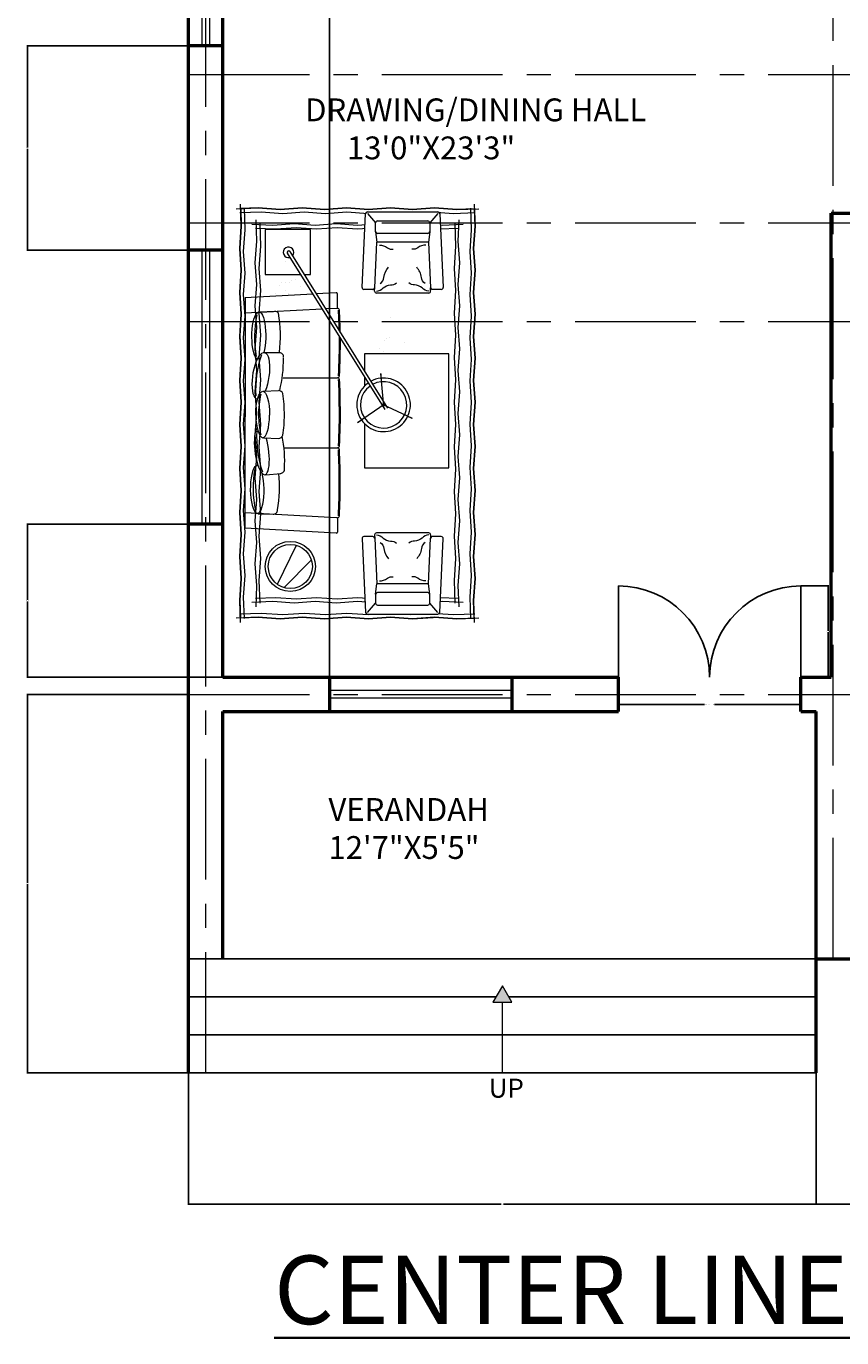
# Model space of a CAD drawing. Units: inches. Extents: x 10696 to 11614, y 5787 to 6498.
# Tile 6 of 9: x 11123 to 11338, y 5787 to 6132. Entities that reach past the tile are written whole.
import ezdxf

# ---------------------------------------------------------------- set-up
doc = ezdxf.new("R2010")
doc.units = ezdxf.units.IN
doc.set_wipeout_variables(frame=1)
doc.linetypes.add('CENTER', pattern=[50.8, 31.75, -6.35, 6.35, -6.35])
for name, color, linetype, lineweight in [('A-ANNO-DIMS', 2, 'Continuous', 18), ('A-ANNO-SYMB', 2, 'Continuous', 18), ('A-ANNO-TITL', 7, 'Continuous', 35), ('A-AREA-IDEN', 7, 'Continuous', 25), ('A-DOOR', 3, 'Continuous', 25), ('A-FLOR', 7, 'Continuous', 25), ('A-FLOR-STRS', 7, 'Continuous', 25), ('A-FURN', 8, 'Continuous', 18), ('A-GLAZ', 4, 'Continuous', 20), ('A-GRID', 1, 'CENTER', 18), ('A-WALL', 7, 'Continuous', 50)]:
    doc.layers.add(name, color=color, linetype=linetype, lineweight=lineweight)
doc.styles.get("Standard").update_dxf_attribs({"font": 'arial.ttf'})
doc.dimstyles.get("Standard").update_dxf_attribs({"dimtxt": 0.18, "dimasz": 0.18, "dimexe": 0.18, "dimexo": 0.0625, "dimgap": 0.09, "dimtad": 0, "dimtih": 1, "dimtoh": 1, "dimdec": 4, "dimzin": 0, "dimdsep": 46, "dimtxsty": 'Standard', "dimcen": 0.09, "dimadec": 0, "dimazin": 0, "dimtfac": 1, "dimtdec": 4, "dimtofl": 0, "dimtmove": 0, "dimatfit": 3, "dimfxl": 1, "dimtolj": 1, "dimtzin": 0, "dimarcsym": 0})

# ---------------------------------------------------------------- blocks, each defined once
blk = doc.blocks.new('A$C7590614E')
for p, q in [((220, 4135), (46, 4129)), ((46, 4129), (52, 3952)), ((46, 4129), (46, 4129)), ((440, 4119), (220, 4135)), ((660, 4135), (440, 4119)), ((881, 4119), (660, 4135)), ((1101, 4135), (881, 4119)), ((1321, 4119), (1101, 4135)), ((1541, 4135), (1321, 4119)), ((1761, 4119), (1541, 4135)), ((1981, 4135), (1761, 4119)), ((2202, 4119), (1981, 4135)), ((2379, 4126), (2202, 4119)), ((2385, 3952), (2379, 4126)), ((52, 3952), (36, 3732)), ((2369, 3732), (2385, 3952)), ((36, 3732), (52, 3513)), ((2385, 3513), (2369, 3732)), ((496, 3597), (496, 3597)), ((596, 3620), (596, 3620)), ((52, 3513), (36, 3293)), ((553, 3416), (553, 3416)), ((592, 3420), (592, 3420)), ((2369, 3293), (2385, 3513)), ((36, 3293), (52, 3074)), ((765, 3275), (91, 3238)), ((392, 3284), (392, 3284)), ((436, 3366), (436, 3366)), ((454, 3393), (454, 3393)), ((492, 3396), (492, 3396)), ((492, 3308), (492, 3308)), ((526, 3286), (526, 3286)), ((536, 3390), (536, 3390)), ((641, 3347), (641, 3347)), ((741, 3371), (741, 3371)), ((1000, 3288), (799, 3277)), ((1011, 3134), (1011, 3278)), ((2385, 3074), (2369, 3293)), ((91, 3238), (91, 2051)), ((91, 3161), (91, 2051)), ((426, 3262), (426, 3262)), ((52, 3074), (37, 2858)), ((859, 3125), (91, 3084)), ((236, 3098), (385, 3104)), ((374, 3100), (240, 3093)), ((332, 3098), (253, 3094)), ((1010, 3133), (893, 3127)), ((1538, 3041), (1538, 3041)), ((2369, 2854), (2385, 3074)), ((37, 2858), (52, 2635)), ((1479, 2810), (1479, 2810)), ((1496, 2837), (1496, 2837)), ((1535, 2840), (1535, 2840)), ((1683, 2791), (1683, 2791)), ((2385, 2635), (2369, 2854)), ((52, 2635), (36, 2415)), ((276, 2693), (435, 2692)), ((1434, 2729), (1434, 2729)), ((1469, 2706), (1469, 2706)), ((2369, 2415), (2385, 2635)), ((36, 2415), (52, 2196)), ((469, 2441), (1012, 2441)), ((2385, 2196), (2369, 2415)), ((275, 2308), (424, 2314)), ((52, 2196), (36, 1976)), ((2369, 1976), (2385, 2196)), ((36, 1976), (52, 1756)), ((91, 941), (91, 2051)), ((91, 941), (91, 2051)), ((2385, 1756), (2369, 1976)), ((275, 1842), (424, 1836)), ((52, 1756), (36, 1537)), ((478, 1742), (1012, 1742)), ((2369, 1537), (2385, 1756)), ((36, 1537), (52, 1317)), ((296, 1474), (445, 1487)), ((2385, 1317), (2369, 1537)), ((52, 1317), (36, 1098)), ((2369, 1098), (2385, 1317)), ((36, 1098), (52, 878)), ((1001, 1045), (91, 1095)), ((221, 1085), (370, 1080)), ((2385, 878), (2369, 1098)), ((1001, 891), (91, 941)), ((1010, 1045), (1001, 1045)), ((1011, 1045), (1011, 901)), ((52, 878), (36, 659)), ((2369, 659), (2385, 878)), ((36, 659), (52, 439)), ((2385, 439), (2369, 659)), ((52, 439), (36, 220)), ((2369, 220), (2385, 439)), ((36, 220), (43, 46)), ((2376, 43), (2369, 220)), ((43, 46), (220, 52)), ((220, 52), (440, 36)), ((440, 36), (660, 52)), ((660, 52), (881, 36)), ((881, 36), (1101, 52)), ((1101, 52), (1321, 36)), ((1321, 36), (1541, 52)), ((1541, 52), (1761, 36)), ((1761, 36), (1966, 51)), ((1966, 51), (1981, 52)), ((1981, 52), (2202, 36)), ((2202, 36), (2376, 43))]:
    blk.add_line(p, q)
at = {"linetype": 'ByBlock'}
for p, q in [((1474, 2154, 0), (1445, 2485, 0)), ((1474, 2154, 0), (1445, 2485, 0)), ((1450, 2427, 0), (1446, 2481, 0)), ((1487, 2182, 0), (1213, 1991, 0)), ((1487, 2182, 0), (1213, 1991, 0)), ((1456, 2179, 0), (1757, 2037, 0)), ((1456, 2179, 0), (1757, 2037, 0)), ((1261, 2025, 0), (1217, 1994, 0)), ((1705, 2062, 0), (1754, 2039, 0)), ((412, 381), (604, 770)), ((751, 626), (481, 348))]:
    blk.add_line(p, q, dxfattribs=at)
at = {"linetype": 'ByBlock', "flags": 128}
for points in [[(0, 4127), (220, 4135), (440, 4119), (660, 4135), (881, 4119), (1101, 4135), (1321, 4119), (1541, 4135), (1761, 4119), (1981, 4135), (2202, 4119), (2422, 4127)], [(44, 0), (36, 220), (52, 439), (36, 659), (52, 878), (36, 1098), (52, 1317), (36, 1537), (52, 1756), (36, 1976), (52, 2196), (36, 2415), (52, 2635), (36, 2854), (52, 3074), (36, 3293), (52, 3513), (36, 3732), (52, 3952), (44, 4172)], [(39, 4088), (252, 4096), (465, 4080), (678, 4096), (891, 4080), (1104, 4096), (1317, 4080), (1531, 4096), (1744, 4080), (1957, 4096), (2170, 4080), (2383, 4088)], [(83, 39), (75, 254), (91, 470), (75, 685), (91, 901), (75, 1116), (91, 1332), (75, 1547), (91, 1763), (75, 1978), (91, 2194), (75, 2409), (91, 2624), (75, 2840), (91, 3055), (75, 3271), (91, 3486), (75, 3702), (91, 3917), (83, 4133)], [(2339, 4133), (2347, 3917), (2331, 3702), (2347, 3486), (2331, 3271), (2347, 3055), (2331, 2840), (2347, 2624), (2331, 2409), (2347, 2194), (2331, 1978), (2347, 1763), (2331, 1547), (2347, 1332), (2331, 1116), (2347, 901), (2331, 685), (2347, 470), (2331, 254), (2339, 39)], [(2377, 4172), (2385, 3952), (2369, 3732), (2385, 3513), (2369, 3293), (2385, 3074), (2369, 2854), (2385, 2635), (2369, 2415), (2385, 2196), (2369, 1976), (2385, 1756), (2369, 1537), (2385, 1317), (2369, 1098), (2385, 878), (2369, 659), (2385, 439), (2369, 220), (2377, 0)], [(156, 3972), (367, 3964), (578, 3980), (789, 3964), (1000, 3980), (1211, 3964), (1422, 3980), (1633, 3964), (1844, 3980), (2055, 3964), (2266, 3972)], [(200, 156), (208, 370), (192, 584), (208, 799), (192, 1013), (208, 1228), (192, 1442), (208, 1657), (192, 1871), (208, 2086), (192, 2300), (208, 2515), (192, 2729), (208, 2944), (192, 3158), (208, 3373), (192, 3587), (208, 3802), (200, 4016)], [(194, 3933), (398, 3925), (601, 3941), (804, 3925), (1008, 3941), (1211, 3925), (1414, 3941), (1617, 3925), (1821, 3941), (2024, 3925), (2227, 3933)], [(239, 194), (231, 417), (247, 639), (231, 862), (247, 1084), (231, 1307), (247, 1529), (231, 1752), (247, 1975), (231, 2197), (247, 2420), (231, 2642), (247, 2865), (231, 3087), (247, 3310), (231, 3532), (247, 3755), (239, 3977)], [(2183, 3977), (2191, 3755), (2175, 3532), (2191, 3310), (2175, 3087), (2191, 2865), (2175, 2642), (2191, 2420), (2175, 2197), (2191, 1975), (2175, 1752), (2191, 1529), (2175, 1307), (2191, 1084), (2175, 862), (2191, 639), (2175, 417), (2183, 194)], [(2222, 4016), (2214, 3802), (2230, 3587), (2214, 3373), (2230, 3158), (2214, 2944), (2230, 2729), (2214, 2515), (2230, 2300), (2214, 2086), (2230, 1871), (2214, 1657), (2230, 1442), (2214, 1228), (2230, 1013), (2214, 799), (2230, 584), (2214, 370), (2222, 156)], [(2266, 200), (2055, 208), (1844, 192), (1633, 208), (1422, 192), (1211, 208), (1000, 192), (789, 208), (578, 192), (367, 208), (156, 200)], [(2227, 239), (2024, 247), (1821, 231), (1617, 247), (1414, 231), (1211, 247), (1008, 231), (804, 247), (601, 231), (398, 247), (194, 239)], [(2422, 44), (2202, 36), (1981, 52), (1761, 36), (1541, 52), (1321, 36), (1101, 52), (881, 36), (660, 52), (440, 36), (220, 52), (0, 44)], [(2383, 83), (2170, 75), (1957, 91), (1744, 75), (1531, 91), (1317, 75), (1104, 91), (891, 75), (678, 91), (465, 75), (252, 91), (39, 83)]]:
    blk.add_lwpolyline(points, dxfattribs=at)
at = {"linetype": 'ByBlock'}
blk.add_lwpolyline([(678, 3471), (741, 3471), (741, 3921), (291, 3921), (291, 3471), (643, 3471)], dxfattribs=at)
for points in [[(1282, 1984), (1282, 1541), (2122, 1541), (2122, 2681), (1282, 2681), (1282, 2504)], [(1282, 2447), (1282, 2359)]]:
    blk.add_lwpolyline(points)
at = {"linetype": 'ByBlock', "const_width": 10, "elevation": 0}
for points in [[(1450, 2427), (1446, 2481)], [(1261, 2025), (1217, 1994)], [(1705, 2062), (1754, 2039)]]:
    blk.add_lwpolyline(points, dxfattribs=at)
at = {"linetype": 'ByBlock'}
for radius in [250, 220]:
    blk.add_circle((541, 559), radius, dxfattribs=at)
for radius, start, end in [(52.4, 318.5939, 285.3184), (15, 31.9562, 211.9562)]:
    blk.add_arc((523, 3692), radius, start, end, dxfattribs=at)
for centre, radius, start, end in [((1001, 3278), 10, 0, 93.0128), ((1254, 2846), 1070, 168.034, 190.3551), ((-385, 2845), 798, 18.6145, 18.6419), ((387, 3061), 42.5, 33.8407, 92.0223), ((-822, 2855), 1265, 352.6106, 10.4711), ((1011, 3113), 20, 3.7459, 93.0128), ((-4595, 2788), 5626, 1.223, 3.3226), ((-4595, 2788), 5636, 1.0525, 3.3226), ((-4595, 2788), 5626, 356.669, 0.6303), ((-4595, 2788), 5636, 356.669, 0.4637), ((1265, 2321), 1070, 160.9121, 183.2331), ((431, 2650), 42.5, 352.6116, 84.9003), ((-796, 2619), 1269, 346.0345, 0.8134), ((1011, 2421), 20, 3.742, 91.3972), ((1011, 2461), 20, 271.3972, 356.2445), ((-2252, 2185), 3282, 359.485, 4.1508), ((-2252, 2185), 3292, 359.485, 4.1508), ((1293, 2055), 1070, 168.034, 179.2769), ((425, 2271), 42.5, 16.3929, 92.0223), ((-783, 2085), 1265, 359.2714, 9.0059), ((425, 2271), 42.5, 359.7336, 1.1068), ((-4089, 2069), 5120, 356.563, 0.9635), ((-4089, 2069), 5130, 356.563, 0.9635), ((1293, 2094), 1070, 181.3636, 191.966), ((-783, 2065), 1265, 350.9941, 0.1868), ((1275, 1851), 1070, 176.7669, 199.0879), ((425, 1879), 42.5, 267.9777, 343.6071), ((-780, 1606), 1265, 356.7804, 11.4363), ((425, 1879), 42.5, 358.8932, 0.2664), ((1011, 1762), 20, 268.6028, 356.258), ((1011, 1722), 20, 3.7555, 88.6028), ((-4697, 1393), 5727, 356.706, 3.3024), ((-4697, 1393), 5737, 356.706, 3.3024), ((1239, 1338), 1070, 169.6449, 191.966), ((-831, 1350), 1265, 349.6584, 6.1656), ((441, 1530), 42.5, 275.0997, 7.3884), ((-400, 1339), 798, 341.3581, 341.3855), ((371, 1122), 42.5, 267.9777, 0.2664), ((1011, 1065), 20, 266.9872, 356.2541), ((1001, 901), 10, 266.9872, 0)]:
    blk.add_arc(centre, radius, start, end)
at = {"extrusion": (0, 0, -1)}
for centre, major_axis, ratio, start_param, end_param in [((227, 2858), (2, 239), 0.289653, 3.343252, 8.61472), ((248, 2460), (35, 232), 0.342983, 3.115548, 8.511087), ((265, 2068), (2, 239), 0.289653, -1.56819, 1.564113)]:
    blk.add_ellipse(centre, major_axis=major_axis, ratio=ratio, start_param=start_param, end_param=end_param, dxfattribs=at)
at = {"linetype": 'ByBlock', "extrusion": (3.38184e-09, 2.26187e-09, 1)}
for major_axis, start_param, end_param in [((-219, -153, 0), 4.720612, 10.891434), ((-190, -132, 0), 4.729628, 10.883141)]:
    blk.add_ellipse((1472, 2171), major_axis=major_axis, ratio=1, start_param=start_param, end_param=end_param, dxfattribs=at)
for centre, major_axis, start_param, end_param in [((265, 2082), (-2, 239), 1.623473, 4.655635), ((257, 1711), (-31, 237), 0.253375, 5.250818), ((211, 1326), (-2, 239), -0.16583, 5.452765)]:
    blk.add_ellipse(centre, major_axis=major_axis, ratio=0.289653, start_param=start_param, end_param=end_param)
for points in [[(1941, 3334), (1941, 3305), (1940, 3297), (1936, 3292), (1929, 3287), (1929, 3287), (1919, 3286), (1838, 3286), (1732, 3286), (1653, 3286), (1475, 3286), (1400, 3286), (1392, 3288), (1387, 3292), (1383, 3298), (1382, 3305), (1382, 3311), (1383, 3317), (1383, 3329), (1383, 3336), (1378, 3327), (1372, 3323), (1366, 3322), (1359, 3322), (1271, 3323), (1263, 3328), (1263, 3328), (1259, 3334), (1258, 3341), (1258, 3341), (1292, 4079), (1294, 4086), (1297, 4091), (1297, 4091), (1310, 4096), (1316, 4096), (1326, 4096), (1336, 4096), (2002, 4096), (2014, 4096), (2026, 4091), (2032, 4079), (2032, 4070), (2066, 3341), (2061, 3328), (2061, 3328), (2048, 3322), (2028, 3322), (1992, 3322), (1958, 3322), (1951, 3324), (1945, 3327), (1944, 3329)], [(1941, 845), (1941, 874), (1940, 882), (1936, 887), (1929, 892), (1929, 892), (1919, 893), (1838, 893), (1732, 893), (1653, 893), (1475, 893), (1400, 893), (1392, 891), (1387, 887), (1383, 881), (1382, 874), (1382, 868), (1383, 862), (1383, 850), (1383, 843), (1378, 852), (1372, 856), (1366, 857), (1359, 857), (1271, 856), (1263, 851), (1263, 851), (1259, 845), (1258, 838), (1258, 838), (1292, 100), (1294, 93), (1297, 88), (1297, 88), (1310, 83), (1316, 83), (1326, 83), (1336, 83), (2002, 83), (2014, 83), (2026, 88), (2032, 100), (2032, 109), (2066, 838), (2061, 851), (2061, 851), (2048, 857), (2028, 857), (1992, 857), (1958, 857), (1951, 855), (1945, 852), (1944, 850)]]:
    blk.add_wipeout(points).translate(0, 0, 0)
at = {"linetype": 'ByBlock'}
for p, q in [((1258, 3341, 0), (1292, 4079, 0)), ((1310, 4096, 0), (2014, 4096, 0)), ((1310, 4078, 0), (1392, 3988, 0)), ((1310, 4078, 0), (1392, 3988, 0)), ((2014, 4078, 0), (1932, 3988, 0)), ((2014, 4078, 0), (1932, 3988, 0)), ((2032, 4079, 0), (2066, 3341, 0)), ((1392, 3898, 0), (1392, 3988, 0)), ((1392, 3898, 0), (1392, 3988, 0)), ((1410, 4006, 0), (1914, 4006, 0)), ((1410, 4006, 0), (1914, 4006, 0)), ((1932, 3988, 0), (1932, 3898, 0)), ((1932, 3988, 0), (1932, 3898, 0)), ((1392, 3898, 0), (1405, 3792, 0)), ((1392, 3898, 0), (1405, 3792, 0)), ((1914, 3880, 0), (1410, 3880, 0)), ((1914, 3880, 0), (1410, 3880, 0)), ((1932, 3898, 0), (1919, 3792, 0)), ((1932, 3898, 0), (1919, 3792, 0)), ((510, 3684), (1484, 2123)), ((536, 3700), (1510, 2138)), ((1384, 3339, 0), (1405, 3792, 0)), ((1384, 3339, 0), (1405, 3792, 0)), ((1919, 3792, 0), (1405, 3792, 0)), ((1919, 3792, 0), (1405, 3792, 0)), ((1919, 3792, 0), (1940, 3339, 0)), ((1919, 3792, 0), (1940, 3339, 0)), ((1366, 3322, 0), (1276, 3322, 0)), ((1382, 3305, 0), (1384, 3339, 0)), ((1923, 3286, 0), (1400, 3286, 0)), ((1941, 3305, 0), (1940, 3339, 0)), ((2048, 3322, 0), (1958, 3322, 0)), ((1258, 838, 0), (1292, 100, 0)), ((1366, 857, 0), (1276, 857, 0)), ((1382, 874, 0), (1384, 840, 0)), ((1384, 840, 0), (1405, 387, 0)), ((1384, 840, 0), (1405, 387, 0)), ((1923, 893, 0), (1400, 893, 0)), ((1919, 387, 0), (1940, 840, 0)), ((1919, 387, 0), (1940, 840, 0)), ((1941, 874, 0), (1940, 840, 0)), ((2048, 857, 0), (1958, 857, 0)), ((2032, 100, 0), (2066, 838, 0)), ((1392, 281, 0), (1405, 387, 0)), ((1392, 281, 0), (1405, 387, 0)), ((1392, 281, 0), (1392, 191, 0)), ((1392, 281, 0), (1392, 191, 0)), ((1919, 387, 0), (1405, 387, 0)), ((1919, 387, 0), (1405, 387, 0)), ((1914, 299, 0), (1410, 299, 0)), ((1914, 299, 0), (1410, 299, 0)), ((1932, 281, 0), (1919, 387, 0)), ((1932, 281, 0), (1919, 387, 0)), ((1932, 191, 0), (1932, 281, 0)), ((1932, 191, 0), (1932, 281, 0)), ((1310, 101, 0), (1392, 191, 0)), ((1310, 101, 0), (1392, 191, 0)), ((1410, 173, 0), (1914, 173, 0)), ((1410, 173, 0), (1914, 173, 0)), ((2014, 101, 0), (1932, 191, 0)), ((2014, 101, 0), (1932, 191, 0)), ((1310, 83, 0), (2014, 83, 0))]:
    blk.add_line(p, q, dxfattribs=at)
at = {"linetype": 'ByBlock', "elevation": 0}
for points in [[(1430, 3765, -0.157856), (1510, 3738, 0.195258), (1568, 3723, 0.506042)], [(1430, 3765, -0.157856), (1510, 3738, 0.195258), (1568, 3723, 0.506042)], [(1894, 3765, 0.157856), (1813, 3738, -0.195258), (1755, 3723, -0.506042)], [(1894, 3765, 0.157856), (1813, 3738, -0.195258), (1755, 3723, -0.506042)], [(1437, 3380, 0.215808), (1475, 3442, -0.158378), (1521, 3543, -0.75133)], [(1437, 3380, 0.215808), (1475, 3442, -0.158378), (1521, 3543, -0.75133)], [(1886, 3380, -0.215808), (1849, 3442, 0.158378), (1802, 3543, 0.75133)], [(1886, 3380, -0.215808), (1849, 3442, 0.158378), (1802, 3543, 0.75133)], [(1400, 3304, 0.13045), (1468, 3337, -0.166434), (1542, 3367, 0.138962), (1601, 3387, -0.132288)], [(1400, 3304, 0.13045), (1468, 3337, -0.166434), (1542, 3367, 0.138962), (1601, 3387, -0.132288)], [(1923, 3304, -0.13045), (1856, 3337, 0.166434), (1781, 3367, -0.138962), (1723, 3387, 0.132288)], [(1923, 3304, -0.13045), (1856, 3337, 0.166434), (1781, 3367, -0.138962), (1723, 3387, 0.132288)], [(1400, 875, -0.13045), (1468, 842, 0.166434), (1542, 812, -0.138962), (1601, 792, 0.132288)], [(1400, 875, -0.13045), (1468, 842, 0.166434), (1542, 812, -0.138962), (1601, 792, 0.132288)], [(1437, 799, -0.215808), (1475, 737, 0.158378), (1521, 636, 0.75133)], [(1437, 799, -0.215808), (1475, 737, 0.158378), (1521, 636, 0.75133)], [(1923, 875, 0.13045), (1856, 842, -0.166434), (1781, 812, 0.138962), (1723, 792, -0.132288)], [(1923, 875, 0.13045), (1856, 842, -0.166434), (1781, 812, 0.138962), (1723, 792, -0.132288)], [(1886, 799, 0.215808), (1849, 737, -0.158378), (1802, 636, -0.75133)], [(1886, 799, 0.215808), (1849, 737, -0.158378), (1802, 636, -0.75133)], [(1430, 414, 0.157856), (1510, 441, -0.195258), (1568, 456, -0.506042)], [(1430, 414, 0.157856), (1510, 441, -0.195258), (1568, 456, -0.506042)], [(1894, 414, -0.157856), (1813, 441, 0.195258), (1755, 456, 0.506042)], [(1894, 414, -0.157856), (1813, 441, 0.195258), (1755, 456, 0.506042)]]:
    blk.add_lwpolyline(points, format="xyb", dxfattribs=at)
at = {"linetype": 'ByBlock'}
for centre, start, end in [((1310, 4078, 0), 90, 177.337), ((2014, 4078, 0), 2.663, 90), ((1410, 3988, 0), 90, 180), ((1410, 3988, 0), 90, 180), ((1914, 3988, 0), 0, 90), ((1914, 3988, 0), 0, 90), ((1410, 3898, 0), 180, 270), ((1410, 3898, 0), 180, 270), ((1914, 3898, 0), 270, 0), ((1914, 3898, 0), 270, 0), ((1276, 3340, 0), 177.337, 270), ((1366, 3340, 0), 270, 357.337), ((1400, 3304, 0), 177.337, 270), ((1923, 3304, 0), 270, 2.663), ((1958, 3340, 0), 182.663, 270), ((2048, 3340, 0), 270, 2.663), ((1276, 839, 0), 90, 182.663), ((1366, 839, 0), 2.663, 90), ((1400, 875, 0), 90, 182.663), ((1923, 875, 0), 357.337, 90), ((1958, 839, 0), 90, 177.337), ((2048, 839, 0), 357.337, 90), ((1410, 281, 0), 90, 180), ((1410, 281, 0), 90, 180), ((1914, 281, 0), 360, 90), ((1914, 281, 0), 360, 90), ((1410, 191, 0), 180, 270), ((1410, 191, 0), 180, 270), ((1914, 191, 0), 270, 360), ((1914, 191, 0), 270, 360), ((1310, 101, 0), 182.663, 270), ((2014, 101, 0), 270, 357.337)]:
    blk.add_arc(centre, 18, start, end, dxfattribs=at)
blk = doc.blocks.new('DOOR-PAIR-48')
for p, q in [((0, 0), (0, 24)), ((48, 0), (48, 24))]:
    blk.add_line(p, q)
for centre, start, end in [((0, 0), 0, 90), ((48, 0), 90, 180)]:
    blk.add_arc(centre, 24, start, end)
blk = doc.blocks.new('WIN-GLAZ-48')
for p, q in [((0, 48), (0, 0)), ((2, 48), (2, 0))]:
    blk.add_line(p, q)
blk = doc.blocks.new('WIN-GLAZ-72')
for p, q in [((0, 72), (0, 0)), ((2, 72), (2, 0))]:
    blk.add_line(p, q)
blk = doc.blocks.new('*D50')
at = {"layer": 'A-ANNO-DIMS', "color": 0, "lineweight": -2, "transparency": 16777216}
for p, q in [((11278.77, 5961.01), (11278.77, 5953.69)), ((11326.77, 5961.01), (11326.77, 5953.69)), ((11278.95, 5953.87), (11301.45, 5953.87)), ((11326.59, 5953.87), (11304.08, 5953.87))]:
    blk.add_line(p, q, dxfattribs=at)
at = {"layer": 'A-ANNO-DIMS', "color": 0, "transparency": 16777216}
for points in [[(11278.95, 5953.9), (11278.95, 5953.84), (11278.77, 5953.87)], [(11326.59, 5953.9), (11326.59, 5953.84), (11326.77, 5953.87)]]:
    blk.add_solid(points, dxfattribs=at)
at = {"layer": 'Defpoints', "color": 0, "transparency": 16777216}
for p in [(11278.77, 5961.07), (11326.77, 5961.07), (11326.77, 5953.87)]:
    blk.add_point(p, dxfattribs=at)
at = {"layer": 'A-ANNO-DIMS', "color": 0, "transparency": 16777216, "insert": (11302.77, 5953.87), "char_height": 0.18, "attachment_point": 5}
blk.add_mtext('\\A1;ENTRY PAIR 48 TYP.', dxfattribs=at)
blk = doc.blocks.new('*D51')
at = {"layer": 'A-ANNO-DIMS', "color": 0, "lineweight": -2, "transparency": 16777216}
for p, q in [((11326.83, 5985.07), (11334.15, 5985.07)), ((11333.97, 5984.89), (11333.97, 5973.25)), ((11333.97, 5961.25), (11333.97, 5972.89)), ((11326.83, 5961.07), (11334.15, 5961.07))]:
    blk.add_line(p, q, dxfattribs=at)
at = {"layer": 'A-ANNO-DIMS', "color": 0, "transparency": 16777216}
for points in [[(11333.94, 5984.89), (11334, 5984.89), (11333.97, 5985.07)], [(11333.94, 5961.25), (11334, 5961.25), (11333.97, 5961.07)]]:
    blk.add_solid(points, dxfattribs=at)
at = {"layer": 'Defpoints', "color": 0, "transparency": 16777216}
for p in [(11326.77, 5985.07), (11333.97, 5985.07), (11326.77, 5961.07)]:
    blk.add_point(p, dxfattribs=at)
at = {"layer": 'A-ANNO-DIMS', "color": 0, "transparency": 16777216, "insert": (11333.97, 5973.07), "char_height": 0.18, "attachment_point": 5}
blk.add_mtext('\\A1;24 TYP.', dxfattribs=at)
blk = doc.blocks.new('*D72')
at = {"layer": 'A-ANNO-DIMS', "color": 0, "lineweight": -2, "transparency": 16777216}
for p, q in [((11165.7, 5956.57), (11123.18, 5956.57)), ((11123.36, 5956.39), (11123.36, 5907)), ((11123.36, 5857.25), (11123.36, 5906.64)), ((11165.7, 5857.07), (11123.18, 5857.07))]:
    blk.add_line(p, q, dxfattribs=at)
at = {"layer": 'A-ANNO-DIMS', "color": 0, "transparency": 16777216}
for points in [[(11123.33, 5956.39), (11123.39, 5956.39), (11123.36, 5956.57)], [(11123.33, 5857.25), (11123.39, 5857.25), (11123.36, 5857.07)]]:
    blk.add_solid(points, dxfattribs=at)
at = {"layer": 'Defpoints', "color": 0, "transparency": 16777216}
for p in [(11123.36, 5956.57), (11165.77, 5956.57), (11165.77, 5857.07)]:
    blk.add_point(p, dxfattribs=at)
at = {"layer": 'A-ANNO-DIMS', "color": 0, "transparency": 16777216, "insert": (11123.36, 5906.82), "char_height": 0.18, "attachment_point": 5}
blk.add_mtext('\\A1;99.5', dxfattribs=at)
blk = doc.blocks.new('*D75')
at = {"layer": 'A-ANNO-DIMS', "color": 0, "lineweight": -2, "transparency": 16777216}
for p, q in [((11165.77, 5857.01), (11165.77, 5822.34)), ((11330.77, 5857.01), (11330.77, 5822.34)), ((11165.95, 5822.52), (11247.99, 5822.52)), ((11330.59, 5822.52), (11248.55, 5822.52))]:
    blk.add_line(p, q, dxfattribs=at)
at = {"layer": 'A-ANNO-DIMS', "color": 0, "transparency": 16777216}
for points in [[(11165.95, 5822.55), (11165.95, 5822.49), (11165.77, 5822.52)], [(11330.59, 5822.55), (11330.59, 5822.49), (11330.77, 5822.52)]]:
    blk.add_solid(points, dxfattribs=at)
at = {"layer": 'Defpoints', "color": 0, "transparency": 16777216}
for p in [(11165.77, 5857.07), (11330.77, 5857.07), (11330.77, 5822.52)]:
    blk.add_point(p, dxfattribs=at)
at = {"layer": 'A-ANNO-DIMS', "color": 0, "transparency": 16777216, "insert": (11248.27, 5822.52), "char_height": 0.18, "attachment_point": 5}
blk.add_mtext('\\A1;165', dxfattribs=at)
blk = doc.blocks.new('*D76')
at = {"layer": 'A-ANNO-DIMS', "color": 0, "lineweight": -2, "transparency": 16777216}
for p, q in [((11330.77, 5887.01), (11330.77, 5822.34)), ((11492.77, 5887.01), (11492.77, 5822.34)), ((11330.95, 5822.52), (11411.49, 5822.52)), ((11492.59, 5822.52), (11412.05, 5822.52))]:
    blk.add_line(p, q, dxfattribs=at)
at = {"layer": 'A-ANNO-DIMS', "color": 0, "transparency": 16777216}
for points in [[(11330.95, 5822.55), (11330.95, 5822.49), (11330.77, 5822.52)], [(11492.59, 5822.55), (11492.59, 5822.49), (11492.77, 5822.52)]]:
    blk.add_solid(points, dxfattribs=at)
at = {"layer": 'Defpoints', "color": 0, "transparency": 16777216}
for p in [(11330.77, 5887.07), (11492.77, 5887.07), (11492.77, 5822.52)]:
    blk.add_point(p, dxfattribs=at)
at = {"layer": 'A-ANNO-DIMS', "color": 0, "transparency": 16777216, "insert": (11411.77, 5822.52), "char_height": 0.18, "attachment_point": 5}
blk.add_mtext('\\A1;162', dxfattribs=at)
blk = doc.blocks.new('*D92')
at = {"layer": 'A-ANNO-DIMS', "color": 0, "lineweight": -2, "transparency": 16777216}
for p, q in [((11165.7, 6001.33), (11123.18, 6001.33)), ((11123.36, 6001.15), (11123.36, 5981.38)), ((11123.36, 5961.25), (11123.36, 5981.02)), ((11174.7, 5961.07), (11123.18, 5961.07))]:
    blk.add_line(p, q, dxfattribs=at)
at = {"layer": 'A-ANNO-DIMS', "color": 0, "transparency": 16777216}
for points in [[(11123.33, 6001.15), (11123.39, 6001.15), (11123.36, 6001.33)], [(11123.33, 5961.25), (11123.39, 5961.25), (11123.36, 5961.07)]]:
    blk.add_solid(points, dxfattribs=at)
at = {"layer": 'Defpoints', "color": 0, "transparency": 16777216}
for p in [(11123.36, 6001.33), (11165.77, 6001.33), (11174.77, 5961.07)]:
    blk.add_point(p, dxfattribs=at)
at = {"layer": 'A-ANNO-DIMS', "color": 0, "transparency": 16777216, "insert": (11123.36, 5981.2), "char_height": 0.18, "attachment_point": 5}
blk.add_mtext('\\A1;40.26', dxfattribs=at)
blk = doc.blocks.new('*D93')
at = {"layer": 'A-ANNO-DIMS', "color": 0, "lineweight": -2, "transparency": 16777216}
for p, q in [((11165.7, 6127.06), (11123.18, 6127.06)), ((11123.36, 6126.88), (11123.36, 6100.38)), ((11123.36, 6073.51), (11123.36, 6100.01)), ((11165.7, 6073.33), (11123.18, 6073.33))]:
    blk.add_line(p, q, dxfattribs=at)
at = {"layer": 'A-ANNO-DIMS', "color": 0, "transparency": 16777216}
for points in [[(11123.33, 6126.88), (11123.39, 6126.88), (11123.36, 6127.06)], [(11123.33, 6073.51), (11123.39, 6073.51), (11123.36, 6073.33)]]:
    blk.add_solid(points, dxfattribs=at)
at = {"layer": 'Defpoints', "color": 0, "transparency": 16777216}
for p in [(11123.36, 6127.06), (11165.77, 6127.06), (11165.77, 6073.33)]:
    blk.add_point(p, dxfattribs=at)
at = {"layer": 'A-ANNO-DIMS', "color": 0, "transparency": 16777216, "insert": (11123.36, 6100.19), "char_height": 0.18, "attachment_point": 5}
blk.add_mtext('\\A1;53.72', dxfattribs=at)
blk = doc.blocks.new('*D95')
at = {"layer": 'A-ANNO-DIMS', "color": 0, "lineweight": -2, "transparency": 16777216}
for p, q in [((11174.77, 5961.13), (11174.77, 6497.62)), ((11174.95, 6497.44), (11188.55, 6497.44)), ((11202.59, 6497.44), (11188.99, 6497.44)), ((11202.77, 5961.13), (11202.77, 6497.62))]:
    blk.add_line(p, q, dxfattribs=at)
at = {"layer": 'A-ANNO-DIMS', "color": 0, "transparency": 16777216}
for points in [[(11174.95, 6497.47), (11174.95, 6497.41), (11174.77, 6497.44)], [(11202.59, 6497.47), (11202.59, 6497.41), (11202.77, 6497.44)]]:
    blk.add_solid(points, dxfattribs=at)
at = {"layer": 'Defpoints', "color": 0, "transparency": 16777216}
for p in [(11202.77, 6497.44), (11174.77, 5961.07), (11202.77, 5961.07)]:
    blk.add_point(p, dxfattribs=at)
at = {"layer": 'A-ANNO-DIMS', "color": 0, "transparency": 16777216, "insert": (11188.77, 6497.44), "char_height": 0.18, "attachment_point": 5}
blk.add_mtext('\\A1;28', dxfattribs=at)

msp = doc.modelspace()

# ---------------------------------------------------------------- hatches: boundary and pattern name
at = {"layer": 'A-ANNO-SYMB'}
h = msp.add_hatch(color=256, dxfattribs=at)
h.dxf.hatch_style = 1
h.paths.add_polyline_path([(11248.267, 5879.918), (11245.801, 5875.646), (11250.734, 5875.646)])

# ---------------------------------------------------------------- linework, layer by layer
msp.add_line((11248.267, 5857.07), (11248.267, 5875.646), dxfattribs=at)
msp.add_lwpolyline([(11248.267, 5879.918), (11245.801, 5875.646), (11250.734, 5875.646)], close=True, dxfattribs=at)
at = {"layer": 'A-FLOR'}
msp.add_line((11165.767, 5887.07), (11330.767, 5887.07), dxfattribs=at)
at = {"layer": 'A-FLOR-STRS'}
for p, q in [((11165.767, 5877.07), (11246.623, 5877.07)), ((11249.912, 5877.07), (11330.767, 5877.07)), ((11165.767, 5867.07), (11330.767, 5867.07)), ((11165.767, 5857.07), (11330.767, 5857.07))]:
    msp.add_line(p, q, dxfattribs=at)
at = {"layer": 'A-GRID'}
for p, q in [((11170.267, 5857.07), (11170.267, 6426.679)), ((11335.267, 5887.07), (11335.267, 6426.679)), ((11165.767, 6119.57), (11554.26, 6119.57)), ((11165.767, 5956.57), (11554.26, 5956.57))]:
    msp.add_line(p, q, dxfattribs=at)
at = {"layer": 'A-WALL'}
for p, q in [((11165.767, 5857.07), (11165.767, 6267.869)), ((11174.767, 5961.07), (11174.767, 6267.869)), ((11174.767, 6127.055), (11165.767, 6127.055)), ((11334.767, 6083.07), (11343.767, 6083.07)), ((11334.767, 5961.07), (11334.767, 6083.07)), ((11174.767, 6073.333), (11165.767, 6073.333)), ((11174.767, 6001.333), (11165.767, 6001.333)), ((11174.767, 5961.07), (11278.767, 5961.07)), ((11202.767, 5961.07), (11202.767, 5952.07)), ((11250.767, 5961.07), (11250.767, 5952.07)), ((11278.767, 5952.07), (11278.767, 5961.07)), ((11326.767, 5961.07), (11334.767, 5961.07)), ((11326.767, 5952.07), (11326.767, 5961.07)), ((11174.767, 5952.07), (11278.767, 5952.07)), ((11174.767, 5887.07), (11174.767, 5952.07)), ((11326.767, 5952.07), (11330.767, 5952.07)), ((11330.767, 5857.07), (11330.767, 5952.07)), ((11330.767, 5887.07), (11492.767, 5887.07))]:
    msp.add_line(p, q, dxfattribs=at)

# ---------------------------------------------------------------- block references
at = {"layer": 'A-DOOR'}
msp.add_blockref('DOOR-PAIR-48', (11278.767, 5961.07), dxfattribs=at)
at = {"layer": 'A-FURN', "xscale": 0.0263548390649643, "yscale": 0.0263548390649643, "zscale": 0.0263548390649643}
msp.add_blockref('A$C7590614E', (11178.241, 5975.473), dxfattribs=at)
at = {"layer": 'A-GLAZ'}
for p in [(11169.267, 6127.055), (11169.267, 6001.333)]:
    msp.add_blockref('WIN-GLAZ-72', p, dxfattribs=at)
at = {"layer": 'A-GLAZ', "rotation": 269.9999999999871}
msp.add_blockref('WIN-GLAZ-48', (11202.767, 5957.57), dxfattribs=at)

# ---------------------------------------------------------------- texts
at = {"layer": 'A-ANNO-SYMB', "insert": (11244.68, 5855.539), "char_height": 5, "attachment_point": 1}
msp.add_mtext_dynamic_manual_height_columns('UP', width=19.19633, gutter_width=12.5, heights=[0], dxfattribs=at)
at = {"layer": 'A-ANNO-TITL', "insert": (11188.246, 5809.021), "char_height": 18, "attachment_point": 1}
msp.add_mtext_dynamic_manual_height_columns('{\\LCENTER LINE DIAGRAM}', width=353.25298, gutter_width=12.5, heights=[0], dxfattribs=at)
at = {"layer": 'A-AREA-IDEN', "char_height": 6, "attachment_point": 1}
for s, width, insert in [('DRAWING/DINING HALL\\P      13\'0"X23\'3"', 143.58411, (11196.392, 6113.237)), ('VERANDAH\\P12\'7"X5\'5"', 76.52537, (11202.529, 5929.31))]:
    msp.add_mtext_dynamic_manual_height_columns(s, width=width, gutter_width=12.5, heights=[0], dxfattribs=dict(at, insert=insert))

# ---------------------------------------------------------------- dimensions: what is measured, and where the dimension line sits
at = {"layer": 'A-ANNO-DIMS'}
for base, p1, p2, override, picture, middle in [((11123.364, 6127.055), (11165.767, 6073.333), (11165.767, 6127.055), {"dimdec": 2, "dimlfac": 1, "dimrnd": 0, "dimzin": 0, "dimdsep": 46, "dimlunit": 2}, '*D93', (11123.364, 6100.194)), ((11123.364, 6001.333), (11174.767, 5961.07), (11165.767, 6001.333), {"dimdec": 2, "dimlfac": 1, "dimrnd": 0, "dimzin": 0, "dimdsep": 46, "dimlunit": 2}, '*D92', (11123.364, 5981.202)), ((11123.364, 5956.57), (11165.767, 5857.07), (11165.767, 5956.57), {"dimdec": 1, "dimlfac": 1, "dimrnd": 0, "dimzin": 0, "dimdsep": 46, "dimlunit": 2}, '*D72', (11123.364, 5906.82))]:
    dim = msp.add_linear_dim(base=base, p1=p1, p2=p2, angle=90, dimstyle='Standard', override=override, dxfattribs=at)
    dim.commit()
    dim.dimension.update_dxf_attribs({"geometry": picture, "text_midpoint": middle})
dim = msp.add_linear_dim(base=(11333.967, 5985.07), p1=(11326.767, 5961.07), p2=(11326.767, 5985.07), angle=90, text='<> TYP.', dimstyle='Standard', override={"dimdec": 0, "dimlfac": 1, "dimrnd": 0, "dimzin": 0, "dimdsep": 46, "dimlunit": 2}, dxfattribs=at)
dim.commit()
dim.dimension.update_dxf_attribs({"geometry": '*D51', "text_midpoint": (11333.967, 5973.07)})
dim = msp.add_linear_dim(base=(11326.767, 5953.87), p1=(11278.767, 5961.07), p2=(11326.767, 5961.07), text='ENTRY PAIR <> TYP.', dimstyle='Standard', override={"dimdec": 0, "dimlfac": 1, "dimrnd": 0, "dimzin": 0, "dimdsep": 46, "dimlunit": 2}, dxfattribs=at)
dim.commit()
dim.dimension.update_dxf_attribs({"geometry": '*D50', "text_midpoint": (11302.767, 5953.87)})
for base, p1, p2, picture, middle in [((11492.767, 5822.52), (11330.767, 5887.07), (11492.767, 5887.07), '*D76', (11411.767, 5822.52)), ((11330.767, 5822.52), (11165.767, 5857.07), (11330.767, 5857.07), '*D75', (11248.267, 5822.52))]:
    dim = msp.add_linear_dim(base=base, p1=p1, p2=p2, dimstyle='Standard', override={"dimdec": 0, "dimlfac": 1, "dimrnd": 0, "dimzin": 0, "dimdsep": 46, "dimlunit": 2}, dxfattribs=at)
    dim.commit()
    dim.dimension.update_dxf_attribs({"geometry": picture, "text_midpoint": middle})

# ---------------------------------------------------------------- next in the draw order: linework, layer by layer
at = {"layer": 'A-GRID'}
for p, q in [((11165.767, 6080.57), (11554.26, 6080.57)), ((11165.767, 6054.57), (11554.26, 6054.57))]:
    msp.add_line(p, q, dxfattribs=at)

# ---------------------------------------------------------------- next in the draw order: dimensions: what is measured, and where the dimension line sits
at = {"layer": 'A-ANNO-DIMS'}
dim = msp.add_linear_dim(base=(11202.767, 6497.443), p1=(11174.767, 5961.07), p2=(11202.767, 5961.07), dimstyle='Standard', override={"dimdec": 0, "dimlfac": 1, "dimrnd": 0, "dimzin": 0, "dimdsep": 46, "dimlunit": 2}, dxfattribs=at)
dim.commit()
dim.dimension.update_dxf_attribs({"geometry": '*D95', "text_midpoint": (11188.767, 6497.443)})

doc.saveas('drawing.dxf')
